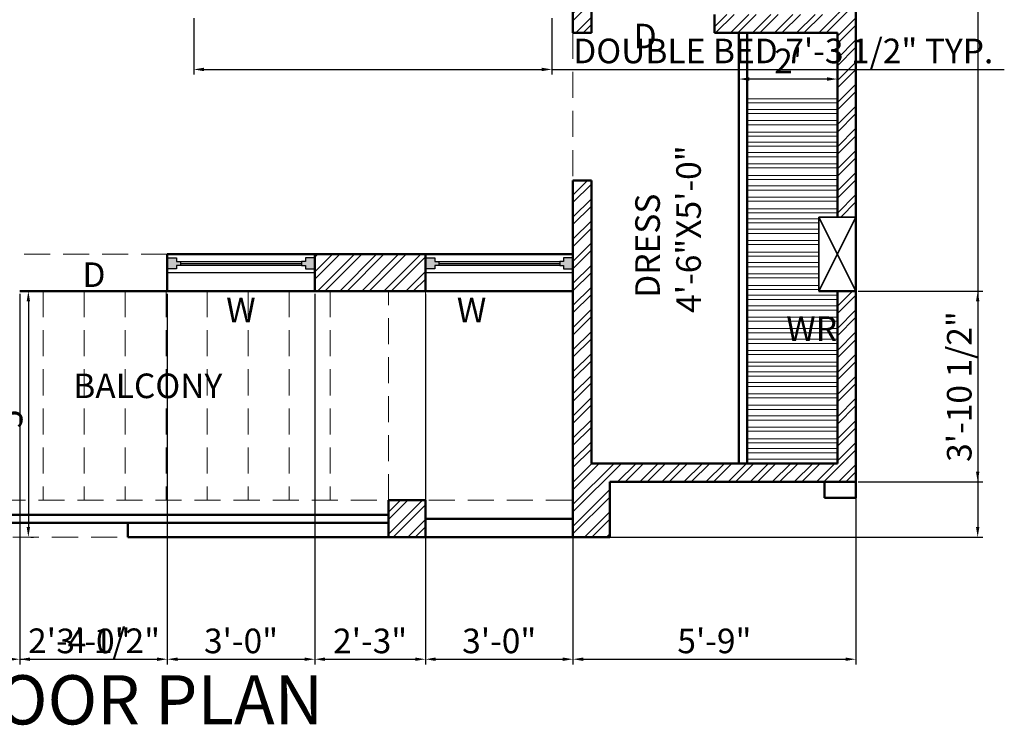
# Model space of a CAD drawing. Units: millimetres. Extents: x 67033 to 68301, y 155969 to 157209.
# Tile 11 of 17: x 67633 to 67874, y 156517 to 156689. Entities that reach past the tile are written whole.
import ezdxf

# ---------------------------------------------------------------- set-up
doc = ezdxf.new("R2010")
doc.units = ezdxf.units.MM
doc.linetypes.add('HIDDEN', pattern=[9.525, 6.35, -3.175])
for name, color, linetype, lineweight in [('A-ANNO-DIMS', 2, 'Continuous', 18), ('A-ANNO-TEXT', 7, 'Continuous', 18), ('A-AREA-IDEN', 3, 'Continuous', 18), ('A-COLS', 3, 'Continuous', 35), ('A-FLOR-OVHD', 1, 'HIDDEN', 18), ('A-FURN', 8, 'Continuous', 18), ('A-GLAZ', 4, 'Continuous', 25), ('A-WALL', 7, 'Continuous', 50), ('A-WALL-PATT', 8, 'Continuous', 13)]:
    doc.layers.add(name, color=color, linetype=linetype, lineweight=lineweight)
doc.styles.get("Standard").update_dxf_attribs({"font": 'arial.ttf'})
doc.dimstyles.new('ISO-25', dxfattribs={"dimtxt": 6, "dimasz": 2.5, "dimexe": 1.25, "dimexo": 0.625, "dimtad": 1, "dimdec": 0, "dimlunit": 3, "dimtxsty": 'Standard', "dimcen": 2.5, "dimadec": 0, "dimazin": 0, "dimtfac": 1, "dimtdec": 0, "dimtmove": 0, "dimatfit": 3, "dimfxl": 1, "dimarcsym": 0})
pattern_1 = [(45, (429.8785, 0), (-2.69407684, 2.69407684), []), (45, (431.6745, 0), (-2.69407684, 2.69407684), [])]

# ---------------------------------------------------------------- blocks, each defined once
blk = doc.blocks.new('*D37')
at = {"layer": 'A-ANNO-DIMS', "color": 0, "lineweight": -2, "transparency": 16777216}
for p, q in [((67636.06, 156622.49), (67636.68, 156622.49)), ((67635.43, 156619.99), (67635.43, 156564.99)), ((67636.06, 156562.49), (67636.68, 156562.49))]:
    blk.add_line(p, q, dxfattribs=at)
at = {"layer": 'A-ANNO-DIMS', "color": 0, "transparency": 16777216}
for points in [[(67635.02, 156619.99), (67635.85, 156619.99), (67635.43, 156622.49)], [(67635.02, 156564.99), (67635.85, 156564.99), (67635.43, 156562.49)]]:
    blk.add_solid(points, dxfattribs=at)
at = {"layer": 'Defpoints', "color": 0, "transparency": 16777216}
for p in [(67635.43, 156622.49), (67635.43, 156562.49), (67635.43, 156562.49)]:
    blk.add_point(p, dxfattribs=at)
at = {"layer": 'A-ANNO-DIMS', "color": 0, "transparency": 16777216, "insert": (67631.76, 156592.49), "char_height": 6, "attachment_point": 5, "rotation": 90}
blk.add_mtext("5'", dxfattribs=at)
blk = doc.blocks.new('*D41')
at = {"layer": 'A-ANNO-DIMS', "color": 0, "lineweight": -2, "transparency": 16777216}
for p, q in [((67808.82, 156675.94), (67808.82, 156672.97)), ((67832.82, 156675.94), (67832.82, 156672.97)), ((67830.32, 156674.22), (67811.32, 156674.22))]:
    blk.add_line(p, q, dxfattribs=at)
at = {"layer": 'A-ANNO-DIMS', "color": 0, "transparency": 16777216}
for points in [[(67811.32, 156674.64), (67811.32, 156673.8), (67808.82, 156674.22)], [(67830.32, 156674.64), (67830.32, 156673.8), (67832.82, 156674.22)]]:
    blk.add_solid(points, dxfattribs=at)
at = {"layer": 'Defpoints', "color": 0, "transparency": 16777216}
for p in [(67808.82, 156676.57), (67832.82, 156676.57), (67808.82, 156674.22)]:
    blk.add_point(p, dxfattribs=at)
at = {"layer": 'A-ANNO-DIMS', "color": 0, "transparency": 16777216, "insert": (67820.82, 156677.86), "char_height": 6, "attachment_point": 5}
blk.add_mtext("2'", dxfattribs=at)
blk = doc.blocks.new('WIN-900')
for p, q in [((3.67, 3.22), (33.2, 3.22)), ((3.67, 2.74), (33.2, 2.74)), ((33.2, 2.27), (3.67, 2.27))]:
    blk.add_line(p, q)
blk.add_lwpolyline([(0.44, 4.99), (36.44, 4.99), (36.44, 0.49), (0.44, 0.49)], close=True)
for points in [[(0.44, 4.09), (2.73, 4.09), (2.73, 3.22), (3.67, 3.22), (3.67, 2.27), (2.73, 2.27), (2.73, 1.4), (0.44, 1.4)], [(36.44, 4.09), (34.14, 4.09), (34.14, 3.22), (33.2, 3.22), (33.2, 2.27), (34.14, 2.27), (34.14, 1.4), (36.44, 1.4)]]:
    blk.add_lwpolyline(points)
blk = doc.blocks.new('COLUMN-230x460')
for p, q in [((0.44, 17.99), (9.44, -0.01)), ((9.44, 17.99), (0.44, -0.01))]:
    blk.add_line(p, q)
blk.add_lwpolyline([(0.44, 17.99), (9.44, 17.99), (9.44, -0.01), (0.44, -0.01)], close=True)
blk = doc.blocks.new('*D57')
at = {"layer": 'A-ANNO-DIMS', "color": 0, "lineweight": -2, "transparency": 16777216}
for p, q in [((67675.78, 156689.05), (67675.78, 156675.31)), ((67763.19, 156689.05), (67763.19, 156675.31)), ((67678.28, 156676.56), (67760.69, 156676.56)), ((67763.19, 156676.56), (67873.56, 156676.56))]:
    blk.add_line(p, q, dxfattribs=at)
at = {"layer": 'A-ANNO-DIMS', "color": 0, "transparency": 16777216}
for points in [[(67678.28, 156676.98), (67678.28, 156676.14), (67675.78, 156676.56)], [(67760.69, 156676.98), (67760.69, 156676.14), (67763.19, 156676.56)]]:
    blk.add_solid(points, dxfattribs=at)
at = {"layer": 'Defpoints', "color": 0, "transparency": 16777216}
for p in [(67675.78, 156689.67), (67763.19, 156689.67), (67763.19, 156676.56)]:
    blk.add_point(p, dxfattribs=at)
at = {"layer": 'A-ANNO-DIMS', "color": 0, "transparency": 16777216, "insert": (67819.62, 156680.29), "char_height": 6, "attachment_point": 5}
blk.add_mtext('DOUBLE BED 7\'-3 1/2" TYP.', dxfattribs=at)
blk = doc.blocks.new('*D105')
at = {"layer": 'A-ANNO-DIMS', "color": 0, "lineweight": -2, "transparency": 16777216}
for p, q in [((67604.81, 156621.86), (67604.81, 156531.49)), ((67633.32, 156621.87), (67633.32, 156531.49)), ((67607.31, 156532.74), (67630.82, 156532.74)), ((67633.32, 156532.74), (67667.1, 156532.74))]:
    blk.add_line(p, q, dxfattribs=at)
at = {"layer": 'A-ANNO-DIMS', "color": 0, "transparency": 16777216}
for points in [[(67607.31, 156533.16), (67607.31, 156532.33), (67604.81, 156532.74)], [(67630.82, 156533.16), (67630.82, 156532.33), (67633.32, 156532.74)]]:
    blk.add_solid(points, dxfattribs=at)
at = {"layer": 'Defpoints', "color": 0, "transparency": 16777216}
for p in [(67604.81, 156622.48), (67633.32, 156622.49), (67633.32, 156532.74)]:
    blk.add_point(p, dxfattribs=at)
at = {"layer": 'A-ANNO-DIMS', "color": 0, "transparency": 16777216, "insert": (67651.46, 156536.47), "char_height": 6, "attachment_point": 5}
blk.add_mtext('2\'-4 1/2"', dxfattribs=at)
blk = doc.blocks.new('*D106')
at = {"layer": 'A-ANNO-DIMS', "color": 0, "lineweight": -2, "transparency": 16777216}
for p, q in [((67633.32, 156621.87), (67633.32, 156531.49)), ((67669.32, 156621.87), (67669.32, 156531.49)), ((67635.82, 156532.74), (67666.82, 156532.74))]:
    blk.add_line(p, q, dxfattribs=at)
at = {"layer": 'A-ANNO-DIMS', "color": 0, "transparency": 16777216}
for points in [[(67635.82, 156533.16), (67635.82, 156532.33), (67633.32, 156532.74)], [(67666.82, 156533.16), (67666.82, 156532.33), (67669.32, 156532.74)]]:
    blk.add_solid(points, dxfattribs=at)
at = {"layer": 'Defpoints', "color": 0, "transparency": 16777216}
for p in [(67633.32, 156622.49), (67669.32, 156622.49), (67669.32, 156532.74)]:
    blk.add_point(p, dxfattribs=at)
at = {"layer": 'A-ANNO-DIMS', "color": 0, "transparency": 16777216, "insert": (67651.32, 156536.43), "char_height": 6, "attachment_point": 5}
blk.add_mtext('3\'-0"', dxfattribs=at)
blk = doc.blocks.new('*D107')
at = {"layer": 'A-ANNO-DIMS', "color": 0, "lineweight": -2, "transparency": 16777216}
for p, q in [((67669.32, 156621.87), (67669.32, 156531.49)), ((67705.32, 156621.87), (67705.32, 156531.49)), ((67671.82, 156532.74), (67702.82, 156532.74))]:
    blk.add_line(p, q, dxfattribs=at)
at = {"layer": 'A-ANNO-DIMS', "color": 0, "transparency": 16777216}
for points in [[(67671.82, 156533.16), (67671.82, 156532.33), (67669.32, 156532.74)], [(67702.82, 156533.16), (67702.82, 156532.33), (67705.32, 156532.74)]]:
    blk.add_solid(points, dxfattribs=at)
at = {"layer": 'Defpoints', "color": 0, "transparency": 16777216}
for p in [(67669.32, 156622.49), (67705.32, 156622.49), (67705.32, 156532.74)]:
    blk.add_point(p, dxfattribs=at)
at = {"layer": 'A-ANNO-DIMS', "color": 0, "transparency": 16777216, "insert": (67687.32, 156536.43), "char_height": 6, "attachment_point": 5}
blk.add_mtext('3\'-0"', dxfattribs=at)
blk = doc.blocks.new('*D108')
at = {"layer": 'A-ANNO-DIMS', "color": 0, "lineweight": -2, "transparency": 16777216}
for p, q in [((67705.32, 156621.87), (67705.32, 156531.49)), ((67732.32, 156621.87), (67732.32, 156531.49)), ((67707.82, 156532.74), (67729.82, 156532.74))]:
    blk.add_line(p, q, dxfattribs=at)
at = {"layer": 'A-ANNO-DIMS', "color": 0, "transparency": 16777216}
for points in [[(67707.82, 156533.16), (67707.82, 156532.33), (67705.32, 156532.74)], [(67729.82, 156533.16), (67729.82, 156532.33), (67732.32, 156532.74)]]:
    blk.add_solid(points, dxfattribs=at)
at = {"layer": 'Defpoints', "color": 0, "transparency": 16777216}
for p in [(67705.32, 156622.49), (67732.32, 156622.49), (67732.32, 156532.74)]:
    blk.add_point(p, dxfattribs=at)
at = {"layer": 'A-ANNO-DIMS', "color": 0, "transparency": 16777216, "insert": (67718.82, 156536.43), "char_height": 6, "attachment_point": 5}
blk.add_mtext('2\'-3"', dxfattribs=at)
blk = doc.blocks.new('*D109')
at = {"layer": 'A-ANNO-DIMS', "color": 0, "lineweight": -2, "transparency": 16777216}
for p, q in [((67732.32, 156621.87), (67732.32, 156531.49)), ((67768.32, 156621.87), (67768.32, 156531.49)), ((67734.82, 156532.74), (67765.82, 156532.74))]:
    blk.add_line(p, q, dxfattribs=at)
at = {"layer": 'A-ANNO-DIMS', "color": 0, "transparency": 16777216}
for points in [[(67734.82, 156533.16), (67734.82, 156532.33), (67732.32, 156532.74)], [(67765.82, 156533.16), (67765.82, 156532.33), (67768.32, 156532.74)]]:
    blk.add_solid(points, dxfattribs=at)
at = {"layer": 'Defpoints', "color": 0, "transparency": 16777216}
for p in [(67732.32, 156622.49), (67768.32, 156622.49), (67768.32, 156532.74)]:
    blk.add_point(p, dxfattribs=at)
at = {"layer": 'A-ANNO-DIMS', "color": 0, "transparency": 16777216, "insert": (67750.32, 156536.43), "char_height": 6, "attachment_point": 5}
blk.add_mtext('3\'-0"', dxfattribs=at)
blk = doc.blocks.new('*D110')
at = {"layer": 'A-ANNO-DIMS', "color": 0, "lineweight": -2, "transparency": 16777216}
for p, q in [((67768.32, 156621.87), (67768.32, 156531.49)), ((67837.32, 156621.87), (67837.32, 156531.49)), ((67770.82, 156532.74), (67834.82, 156532.74))]:
    blk.add_line(p, q, dxfattribs=at)
at = {"layer": 'A-ANNO-DIMS', "color": 0, "transparency": 16777216}
for points in [[(67770.82, 156533.16), (67770.82, 156532.33), (67768.32, 156532.74)], [(67834.82, 156533.16), (67834.82, 156532.33), (67837.32, 156532.74)]]:
    blk.add_solid(points, dxfattribs=at)
at = {"layer": 'Defpoints', "color": 0, "transparency": 16777216}
for p in [(67768.32, 156622.49), (67837.32, 156622.49), (67837.32, 156532.74)]:
    blk.add_point(p, dxfattribs=at)
at = {"layer": 'A-ANNO-DIMS', "color": 0, "transparency": 16777216, "insert": (67802.82, 156536.43), "char_height": 6, "attachment_point": 5}
blk.add_mtext('5\'-9"', dxfattribs=at)
blk = doc.blocks.new('*D112')
at = {"layer": 'A-ANNO-DIMS', "color": 0, "lineweight": -2, "transparency": 16777216}
for p, q in [((67601.44, 157144.49), (67868.32, 157144.49)), ((67867.07, 157141.99), (67867.07, 156564.99)), ((67768.94, 156562.49), (67868.32, 156562.49))]:
    blk.add_line(p, q, dxfattribs=at)
at = {"layer": 'A-ANNO-DIMS', "color": 0, "transparency": 16777216}
for points in [[(67866.65, 157141.99), (67867.48, 157141.99), (67867.07, 157144.49)], [(67866.65, 156564.99), (67867.48, 156564.99), (67867.07, 156562.49)]]:
    blk.add_solid(points, dxfattribs=at)
at = {"layer": 'Defpoints', "color": 0, "transparency": 16777216}
for p in [(67600.82, 157144.49), (67768.32, 156562.49), (67867.07, 156562.49)]:
    blk.add_point(p, dxfattribs=at)
at = {"layer": 'A-ANNO-DIMS', "color": 0, "transparency": 16777216, "insert": (67863.38, 156853.49), "char_height": 6, "attachment_point": 5, "rotation": 90}
blk.add_mtext('48\'-6"', dxfattribs=at)
blk = doc.blocks.new('*D114')
at = {"layer": 'A-ANNO-DIMS', "color": 0, "lineweight": -2, "transparency": 16777216}
for p, q in [((67837.94, 156622.49), (67868.32, 156622.49)), ((67867.07, 156619.99), (67867.07, 156578.49)), ((67837.94, 156575.99), (67868.32, 156575.99))]:
    blk.add_line(p, q, dxfattribs=at)
at = {"layer": 'A-ANNO-DIMS', "color": 0, "transparency": 16777216}
for points in [[(67866.65, 156619.99), (67867.48, 156619.99), (67867.07, 156622.49)], [(67866.65, 156578.49), (67867.48, 156578.49), (67867.07, 156575.99)]]:
    blk.add_solid(points, dxfattribs=at)
at = {"layer": 'Defpoints', "color": 0, "transparency": 16777216}
for p in [(67837.32, 156622.49), (67837.32, 156575.99), (67867.07, 156575.99)]:
    blk.add_point(p, dxfattribs=at)
at = {"layer": 'A-ANNO-DIMS', "color": 0, "transparency": 16777216, "insert": (67863.34, 156599.24), "char_height": 6, "attachment_point": 5, "rotation": 90}
blk.add_mtext('3\'-10 1/2"', dxfattribs=at)

msp = doc.modelspace()

# ---------------------------------------------------------------- hatches: boundary and pattern name
at = {"layer": 'A-GLAZ'}
h = msp.add_hatch(color=256, dxfattribs=at)
h.dxf.hatch_style = 1
h.paths.add_polyline_path([(67672.55, 156629.72), (67671.61, 156629.72), (67671.61, 156630.59), (67669.32, 156630.59), (67669.32, 156627.9), (67671.61, 156627.9), (67671.61, 156628.77), (67672.55, 156628.77)])
h = msp.add_hatch(color=256, dxfattribs=at)
h.dxf.hatch_style = 1
h.paths.add_polyline_path([(67705.32, 156630.59), (67703.02, 156630.59), (67703.02, 156629.72), (67702.08, 156629.72), (67702.08, 156628.77), (67703.02, 156628.77), (67703.02, 156627.9), (67705.32, 156627.9)])
h = msp.add_hatch(color=256, dxfattribs=at)
h.dxf.hatch_style = 1
h.paths.add_polyline_path([(67735.55, 156629.72), (67734.61, 156629.72), (67734.61, 156630.59), (67732.32, 156630.59), (67732.32, 156627.9), (67734.61, 156627.9), (67734.61, 156628.77), (67735.55, 156628.77)])
h = msp.add_hatch(color=256, dxfattribs=at)
h.dxf.hatch_style = 1
h.paths.add_polyline_path([(67768.32, 156630.59), (67766.02, 156630.59), (67766.02, 156629.72), (67765.08, 156629.72), (67765.08, 156628.77), (67766.02, 156628.77), (67766.02, 156627.9), (67768.32, 156627.9)])
at = {"layer": 'A-WALL-PATT'}
h = msp.add_hatch(dxfattribs=at)
h.set_pattern_fill('ANSI32', color=256, scale=0.4)
h.set_pattern_definition(pattern_1)
h.paths.add_polyline_path([(67837.32, 156941.99), (67832.82, 156941.99), (67832.82, 156802.49), (67772.82, 156802.49), (67772.82, 156822.09), (67772.82, 156871.49), (67768.32, 156871.49), (67768.32, 156770.99), (67666.32, 156770.99), (67666.32, 156766.49), (67768.32, 156766.49), (67768.32, 156685.49), (67772.82, 156685.49), (67772.82, 156797.99), (67832.82, 156797.99), (67832.82, 156767.19), (67837.32, 156767.19)])
h = msp.add_hatch(dxfattribs=at)
h.set_pattern_fill('ANSI32', color=256, scale=0.4)
h.set_pattern_definition(pattern_1)
h.paths.add_polyline_path([(67837.32, 156749.19), (67832.82, 156749.19), (67832.82, 156689.99), (67814.5, 156689.99), (67802.82, 156689.99), (67802.82, 156685.49), (67832.82, 156685.49), (67832.82, 156640.49), (67837.32, 156640.49)])
h = msp.add_hatch(dxfattribs=at)
h.set_pattern_fill('ANSI32', color=256, scale=0.4)
h.paths.add_polyline_path([(67777.32, 156575.99), (67837.32, 156575.99), (67837.32, 156622.49), (67832.82, 156622.49), (67832.82, 156580.49), (67772.82, 156580.49), (67772.82, 156649.49), (67768.32, 156649.49), (67768.32, 156562.49), (67777.32, 156562.49)])
h = msp.add_hatch(dxfattribs=at)
h.set_pattern_fill('ANSI32', color=256, scale=0.4)
h.set_pattern_definition(pattern_1)
h.paths.add_polyline_path([(67732.32, 156631.49), (67705.32, 156631.49), (67705.32, 156626.99), (67705.32, 156622.49), (67732.32, 156622.49)])
h = msp.add_hatch(dxfattribs=at)
h.set_pattern_fill('ANSI32', color=256, scale=0.4)
h.paths.add_polyline_path([(67732.32, 156571.49), (67723.32, 156571.49), (67723.32, 156562.49), (67732.32, 156562.49)])

# ---------------------------------------------------------------- linework, layer by layer
at = {"layer": 'A-FLOR-OVHD'}
for p, q in [((67768.32, 156685.49), (67768.32, 156649.49)), ((67669.32, 156631.49), (67633.32, 156631.49)), ((67639.07, 156622.49), (67639.07, 156571.49)), ((67649.07, 156622.49), (67649.07, 156571.49)), ((67659.07, 156622.49), (67659.07, 156571.49)), ((67669.07, 156622.49), (67669.07, 156571.49)), ((67679.07, 156622.49), (67679.07, 156571.49)), ((67689.07, 156622.49), (67689.07, 156571.49)), ((67699.07, 156622.49), (67699.07, 156571.49)), ((67709.07, 156622.49), (67709.07, 156571.49)), ((67723.32, 156571.49), (67723.32, 156622.49)), ((67732.32, 156571.49), (67732.32, 156622.49)), ((67609.32, 156571.49), (67768.32, 156571.49)), ((67498.32, 156562.49), (67732.32, 156562.49))]:
    msp.add_line(p, q, dxfattribs=at)
at = {"layer": 'A-FURN'}
for p, q in [((67810.82, 156669.41), (67832.82, 156669.41)), ((67810.82, 156668.41), (67832.82, 156668.41)), ((67810.82, 156666.82), (67832.82, 156666.82)), ((67810.82, 156665.82), (67832.82, 156665.82)), ((67810.82, 156664.09), (67832.82, 156664.09)), ((67810.82, 156663.09), (67832.82, 156663.09)), ((67810.82, 156661.27), (67832.82, 156661.27)), ((67810.82, 156660.27), (67832.82, 156660.27)), ((67810.82, 156658.86), (67832.82, 156658.86)), ((67810.82, 156657.86), (67832.82, 156657.86)), ((67810.82, 156656.27), (67832.82, 156656.27)), ((67810.82, 156655.27), (67832.82, 156655.27)), ((67810.82, 156653.54), (67832.82, 156653.54)), ((67810.82, 156652.54), (67832.82, 156652.54)), ((67810.82, 156650.72), (67832.82, 156650.72)), ((67810.82, 156649.72), (67832.82, 156649.72)), ((67810.82, 156648.14), (67832.82, 156648.14)), ((67810.82, 156647.14), (67832.82, 156647.14)), ((67810.82, 156645.4), (67832.82, 156645.4)), ((67810.82, 156644.4), (67832.82, 156644.4)), ((67810.82, 156642.59), (67832.82, 156642.59)), ((67810.82, 156641.59), (67832.82, 156641.59)), ((67810.82, 156640.17), (67828.32, 156640.17)), ((67810.82, 156639.17), (67828.32, 156639.17)), ((67810.82, 156637.58), (67828.32, 156637.58)), ((67810.82, 156636.58), (67828.32, 156636.58)), ((67810.82, 156634.85), (67828.32, 156634.85)), ((67810.82, 156633.85), (67828.32, 156633.85)), ((67810.82, 156632.03), (67828.32, 156632.03)), ((67810.82, 156631.03), (67828.32, 156631.03)), ((67810.82, 156629.45), (67828.32, 156629.45)), ((67810.82, 156628.45), (67828.32, 156628.45)), ((67810.82, 156626.71), (67828.32, 156626.71)), ((67810.82, 156625.71), (67828.32, 156625.71)), ((67810.82, 156623.9), (67828.32, 156623.9)), ((67810.82, 156622.9), (67828.32, 156622.9)), ((67810.82, 156621.48), (67832.82, 156621.48)), ((67810.82, 156620.48), (67832.82, 156620.48)), ((67810.82, 156618.9), (67832.82, 156618.9)), ((67810.82, 156617.9), (67832.82, 156617.9)), ((67810.82, 156616.16), (67832.82, 156616.16)), ((67810.82, 156615.16), (67832.82, 156615.16)), ((67810.82, 156613.35), (67832.82, 156613.35)), ((67810.82, 156612.35), (67832.82, 156612.35)), ((67810.82, 156610.76), (67832.82, 156610.76)), ((67810.82, 156609.76), (67832.82, 156609.76)), ((67810.82, 156608.02), (67832.82, 156608.02)), ((67810.82, 156607.02), (67832.82, 156607.02)), ((67810.82, 156605.21), (67832.82, 156605.21)), ((67810.82, 156604.21), (67832.82, 156604.21)), ((67810.82, 156602.79), (67832.82, 156602.79)), ((67810.82, 156601.79), (67832.82, 156601.79)), ((67810.82, 156600.21), (67832.82, 156600.21)), ((67810.82, 156599.21), (67832.82, 156599.21)), ((67810.82, 156597.47), (67832.82, 156597.47)), ((67810.82, 156596.47), (67832.82, 156596.47)), ((67810.82, 156594.66), (67832.82, 156594.66)), ((67810.82, 156593.66), (67832.82, 156593.66)), ((67810.82, 156592.07), (67832.82, 156592.07)), ((67810.82, 156591.07), (67832.82, 156591.07)), ((67810.82, 156589.34), (67832.82, 156589.34)), ((67810.82, 156588.34), (67832.82, 156588.34)), ((67810.82, 156586.52), (67832.82, 156586.52)), ((67810.82, 156585.52), (67832.82, 156585.52)), ((67810.82, 156584.11), (67832.82, 156584.11)), ((67810.82, 156583.11), (67832.82, 156583.11)), ((67810.82, 156581.52), (67832.82, 156581.52)), ((67810.82, 156580.52), (67832.82, 156580.52)), ((67810.82, 156575.97), (67832.82, 156575.97))]:
    msp.add_line(p, q, dxfattribs=at)
at = {"layer": 'A-WALL'}
for p, q in [((67837.32, 157082.99), (67837.32, 156572.08)), ((67772.82, 156797.99), (67772.82, 156685.49)), ((67768.32, 156766.49), (67768.32, 156685.49)), ((67802.82, 156689.99), (67802.82, 156685.49)), ((67768.32, 156685.49), (67772.82, 156685.49)), ((67802.82, 156685.49), (67832.82, 156685.49)), ((67808.82, 156685.49), (67808.82, 156580.49)), ((67810.82, 156685.49), (67810.82, 156580.49)), ((67832.82, 156685.49), (67832.82, 156640.49)), ((67768.32, 156649.49), (67768.32, 156562.49)), ((67768.32, 156649.49), (67772.82, 156649.49)), ((67772.82, 156649.49), (67772.82, 156580.49)), ((67669.32, 156631.49), (67768.32, 156631.49)), ((67669.32, 156631.49), (67669.32, 156622.49)), ((67669.32, 156631.49), (67669.32, 156626.99)), ((67705.32, 156631.49), (67705.32, 156622.49)), ((67705.32, 156631.49), (67705.32, 156626.99)), ((67732.32, 156631.49), (67732.32, 156622.49)), ((67732.32, 156631.49), (67732.32, 156626.99)), ((67768.32, 156631.49), (67768.32, 156626.99)), ((67633.32, 156622.49), (67669.32, 156622.49)), ((67669.32, 156622.49), (67768.32, 156622.49)), ((67828.32, 156622.49), (67837.32, 156622.49)), ((67832.82, 156622.49), (67832.82, 156580.49)), ((67772.82, 156580.49), (67832.82, 156580.49)), ((67777.32, 156575.99), (67837.32, 156575.99)), ((67777.32, 156575.99), (67777.32, 156562.49)), ((67829.67, 156572.08), (67829.67, 156575.99)), ((67837.32, 156572.08), (67829.67, 156572.08)), ((67723.32, 156567.99), (67607.66, 156567.99)), ((67732.32, 156566.99), (67768.32, 156566.99)), ((67723.32, 156565.99), (67605.66, 156565.99)), ((67659.73, 156562.49), (67659.73, 156565.99)), ((67723.32, 156562.49), (67659.73, 156562.49)), ((67732.32, 156562.49), (67768.32, 156562.49)), ((67768.32, 156562.49), (67777.32, 156562.49))]:
    msp.add_line(p, q, dxfattribs=at)
msp.add_lwpolyline([(67732.32, 156562.49), (67723.32, 156562.49), (67723.32, 156571.49), (67732.32, 156571.49)], close=True, dxfattribs=at)

# ---------------------------------------------------------------- block references
at = {"layer": 'A-COLS', "rotation": 180}
msp.add_blockref('COLUMN-230x460', (67837.75, 156640.49), dxfattribs=at)
at = {"layer": 'A-GLAZ'}
for p in [(67668.88, 156626.5), (67731.88, 156626.5)]:
    msp.add_blockref('WIN-900', p, dxfattribs=at)

# ---------------------------------------------------------------- texts
at = {"layer": 'A-ANNO-TEXT', "attachment_point": 1}
for s, width, insert, char_height in [('   D', 19.5287, (67777.61, 156687.7), 6), ('   D', 19.5287, (67643.12, 156629.51), 6), ('   W', 19.5287, (67678.2, 156620.89), 6), ('   W', 19.5287, (67734.48, 156620.88), 6), ('   WR', 19.5287, (67814.85, 156616.36), 6), ('FIRST FLOOR PLAN', 203.6887, (67562.58, 156528.84), 12)]:
    msp.add_mtext_dynamic_manual_height_columns(s, width=width, gutter_width=12.5, heights=[0], dxfattribs=dict(at, insert=insert, char_height=char_height))
at = {"layer": 'A-AREA-IDEN', "insert": (67783.51, 156615.36), "char_height": 6, "attachment_point": 1, "rotation": 90}
msp.add_mtext_dynamic_manual_height_columns('   DRESS\\P 4\'-6"X5\'-0"', width=46.8836, gutter_width=12.5, heights=[0], dxfattribs=at)
at = {"layer": 'A-AREA-IDEN', "insert": (67639.06, 156602.41), "char_height": 6, "attachment_point": 1}
msp.add_mtext_dynamic_manual_height_columns('    BALCONY', width=59.4046, gutter_width=12.5, heights=[0], dxfattribs=at)

# ---------------------------------------------------------------- dimensions: what is measured, and where the dimension line sits
at = {"layer": 'A-ANNO-DIMS'}
for base, p1, p2, override, picture, middle in [((67867.07, 156562.49), (67600.82, 157144.49), (67768.32, 156562.49), {"dimdec": 1, "dimlfac": 1, "dimrnd": 0, "dimzin": 1, "dimdsep": 46, "dimlunit": 4, "dimfrac": 2}, '*D112', (67863.38, 156853.49)), ((67635.43, 156562.49), (67635.43, 156622.49), (67635.43, 156562.49), {"dimclrd": 0, "dimclre": 0, "dimclrt": 0}, '*D37', (67631.76, 156592.49)), ((67867.07, 156575.99), (67837.32, 156622.49), (67837.32, 156575.99), {"dimdec": 1, "dimlfac": 1, "dimrnd": 0, "dimzin": 1, "dimdsep": 46, "dimlunit": 4, "dimfrac": 2}, '*D114', (67863.34, 156599.24))]:
    dim = msp.add_linear_dim(base=base, p1=p1, p2=p2, angle=90, dimstyle='ISO-25', override=override, dxfattribs=at)
    dim.commit()
    dim.dimension.update_dxf_attribs({"geometry": picture, "text_midpoint": middle})
dim = msp.add_linear_dim(base=(67763.19, 156676.56), p1=(67675.78, 156689.67), p2=(67763.19, 156689.67), text='DOUBLE BED <> TYP.', dimstyle='ISO-25', override={"dimdec": 1, "dimrnd": 0, "dimzin": 1, "dimlunit": 4, "dimfrac": 2}, dxfattribs=at)
dim.commit()
dim.dimension.update_dxf_attribs({"geometry": '*D57', "text_midpoint": (67819.62, 156680.29)})
for base, p1, p2, override, picture, middle in [((67808.82, 156674.22), (67832.82, 156676.57), (67808.82, 156676.57), {"dimclrd": 0, "dimclre": 0, "dimclrt": 0}, '*D41', (67820.82, 156677.86)), ((67633.32, 156532.74), (67604.81, 156622.48), (67633.32, 156622.49), {"dimdec": 1, "dimlfac": 1, "dimrnd": 0, "dimzin": 1, "dimdsep": 46, "dimlunit": 4, "dimfrac": 2}, '*D105', (67651.46, 156536.47)), ((67669.32, 156532.74), (67633.32, 156622.49), (67669.32, 156622.49), {"dimdec": 1, "dimlfac": 1, "dimrnd": 0, "dimzin": 1, "dimdsep": 46, "dimlunit": 4, "dimfrac": 2}, '*D106', (67651.32, 156536.43)), ((67705.32, 156532.74), (67669.32, 156622.49), (67705.32, 156622.49), {"dimdec": 1, "dimlfac": 1, "dimrnd": 0, "dimzin": 1, "dimdsep": 46, "dimlunit": 4, "dimfrac": 2}, '*D107', (67687.32, 156536.43)), ((67732.32, 156532.74), (67705.32, 156622.49), (67732.32, 156622.49), {"dimdec": 1, "dimlfac": 1, "dimrnd": 0, "dimzin": 1, "dimdsep": 46, "dimlunit": 4, "dimfrac": 2}, '*D108', (67718.82, 156536.43)), ((67768.32, 156532.74), (67732.32, 156622.49), (67768.32, 156622.49), {"dimdec": 1, "dimlfac": 1, "dimrnd": 0, "dimzin": 1, "dimdsep": 46, "dimlunit": 4, "dimfrac": 2}, '*D109', (67750.32, 156536.43)), ((67837.32, 156532.74), (67768.32, 156622.49), (67837.32, 156622.49), {"dimdec": 1, "dimlfac": 1, "dimrnd": 0, "dimzin": 1, "dimdsep": 46, "dimlunit": 4, "dimfrac": 2}, '*D110', (67802.82, 156536.43))]:
    dim = msp.add_linear_dim(base=base, p1=p1, p2=p2, dimstyle='ISO-25', override=override, dxfattribs=at)
    dim.commit()
    dim.dimension.update_dxf_attribs({"geometry": picture, "text_midpoint": middle})

doc.saveas('drawing.dxf')
